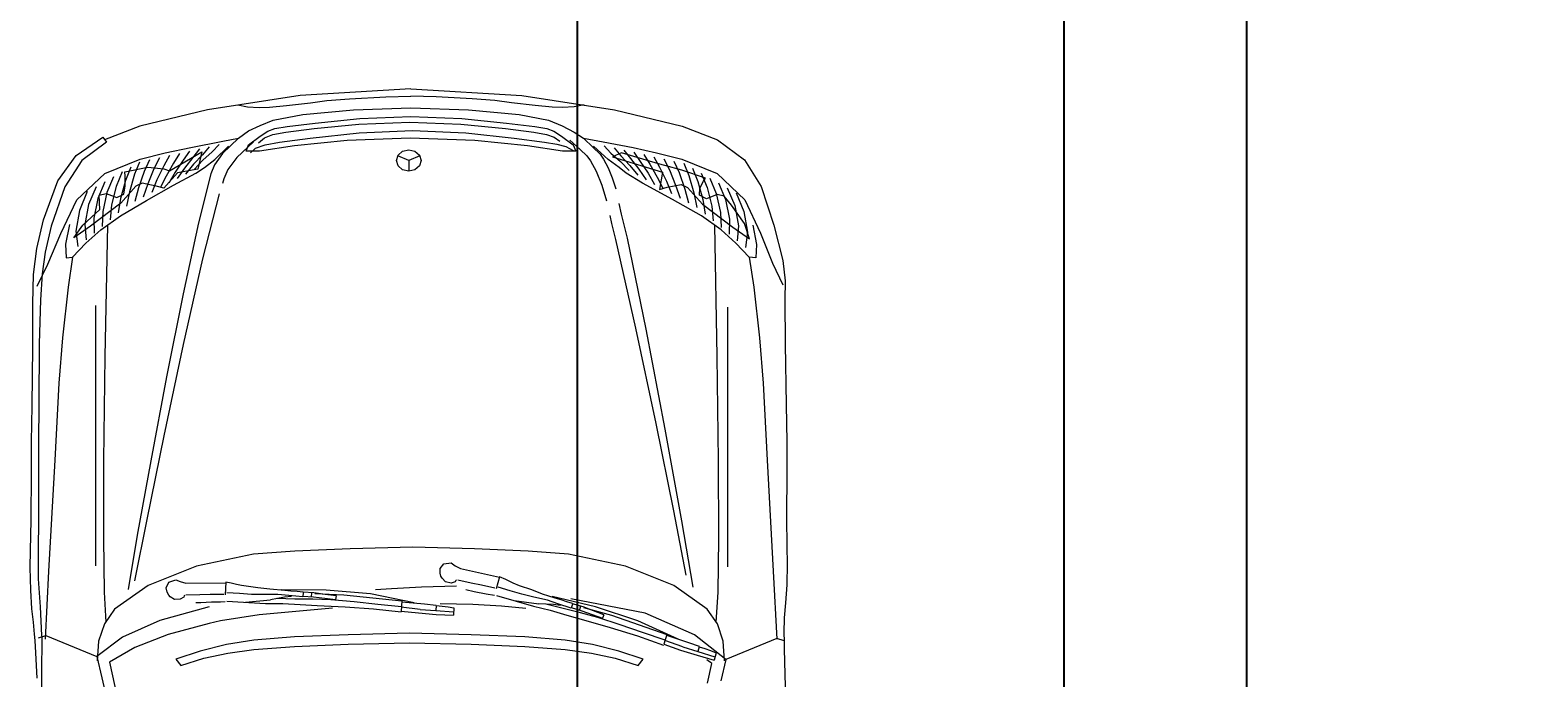
# Model space of a CAD drawing. Units: inches. Extents: x 37 to 706, y -568 to 110.
# Tile 14 of 24: x 452 to 526, y -405 to -373. Entities that reach past the tile are written whole.
import ezdxf

# ---------------------------------------------------------------- set-up
doc = ezdxf.new("R2010")
doc.units = ezdxf.units.IN
doc.header["$MEASUREMENT"] = 0
doc.layers.add('A-ANNO-DIMS', color=2, linetype='Continuous', lineweight=18)
doc.layers.add('A-SITE-VEHI', color=8, linetype='Continuous', lineweight=13)
doc.styles.get("Standard").update_dxf_attribs({"font": 'arial.ttf'})
doc.dimstyles.get("Standard").update_dxf_attribs({"dimtxt": 0.18, "dimasz": 0.18, "dimexe": 0.18, "dimexo": 0.0625, "dimgap": 0.09, "dimtad": 0, "dimtih": 1, "dimtoh": 1, "dimdec": 0, "dimzin": 0, "dimdsep": 46, "dimlunit": 3, "dimtxsty": 'Standard', "dimcen": 0.09, "dimadec": 0, "dimazin": 0, "dimtfac": 1, "dimtdec": 0, "dimtofl": 0, "dimtmove": 0, "dimatfit": 3, "dimfxl": 1, "dimtolj": 1, "dimtzin": 0, "dimarcsym": 0})

# ---------------------------------------------------------------- blocks, each defined once
blk = doc.blocks.new('CAR-SEDAN-PLAN')
for p, q in [((16.648, 91.844), (12.074, 91.146)), ((15.977, 91.359), (17.154, 91.49)), ((22.11, 92.169), (16.648, 91.844)), ((17.154, 91.49), (17.965, 91.597)), ((17.965, 91.597), (19.087, 91.685)), ((19.087, 91.685), (20.868, 91.772)), ((20.868, 91.772), (22.11, 91.812)), ((22.11, 92.169), (27.571, 91.844)), ((23.351, 91.772), (22.11, 91.812)), ((25.132, 91.685), (23.351, 91.772)), ((26.254, 91.597), (25.132, 91.685)), ((27.066, 91.49), (26.254, 91.597)), ((28.242, 91.359), (27.066, 91.49)), ((27.571, 91.844), (32.145, 91.146)), ((12.074, 91.146), (8.74, 90.335)), ((13.57, 91.383), (14.057, 91.284)), ((14.057, 91.284), (14.632, 91.256)), ((14.632, 91.256), (15.142, 91.276)), ((15.142, 91.276), (15.977, 91.359)), ((15.321, 90.633), (16.772, 90.917)), ((16.772, 90.917), (19.278, 91.146)), ((19.278, 91.146), (22.11, 91.24)), ((19.597, 90.705), (22.11, 90.811)), ((22.11, 91.24), (24.942, 91.146)), ((22.11, 90.811), (24.623, 90.705)), ((24.942, 91.146), (27.448, 90.917)), ((27.448, 90.917), (28.898, 90.633)), ((29.077, 91.276), (28.242, 91.359)), ((29.588, 91.256), (29.077, 91.276)), ((30.162, 91.284), (29.588, 91.256)), ((30.649, 91.383), (30.162, 91.284)), ((32.145, 91.146), (35.48, 90.335)), ((8.74, 90.335), (6.996, 89.668)), ((13.606, 89.739), (14.1, 90.1)), ((14.1, 90.1), (14.675, 90.37)), ((14.675, 90.37), (15.321, 90.633)), ((14.678, 89.847), (15.057, 90.081)), ((15.057, 90.081), (15.401, 90.212)), ((15.292, 89.924), (15.945, 90.036)), ((15.401, 90.212), (16, 90.311)), ((15.945, 90.036), (17.338, 90.213)), ((16, 90.311), (17.394, 90.488)), ((17.142, 89.744), (19.563, 89.998)), ((17.338, 90.213), (19.542, 90.43)), ((17.394, 90.488), (19.597, 90.705)), ((19.542, 90.43), (22.055, 90.536)), ((19.563, 89.998), (22.192, 90.123)), ((22.055, 90.536), (24.568, 90.43)), ((22.192, 90.123), (24.809, 89.998)), ((24.568, 90.43), (26.771, 90.213)), ((24.623, 90.705), (26.826, 90.488)), ((24.809, 89.998), (27.204, 89.744)), ((26.771, 90.213), (28.165, 90.036)), ((26.826, 90.488), (28.22, 90.311)), ((28.165, 90.036), (28.798, 89.928)), ((28.22, 90.311), (28.818, 90.212)), ((28.818, 90.212), (29.163, 90.081)), ((28.898, 90.633), (29.564, 90.343)), ((29.163, 90.081), (29.542, 89.847)), ((29.564, 90.343), (30.157, 90.045)), ((30.157, 90.045), (30.614, 89.739)), ((35.48, 90.335), (37.224, 89.668)), ((5.601, 88.894), (6.92, 89.795)), ((7.094, 89.544), (5.88, 88.648)), ((6.92, 89.795), (7.094, 89.544)), ((9.997, 89.025), (11.251, 89.289)), ((11.251, 89.289), (12.829, 89.594)), ((12.166, 89.318), (11.835, 88.927)), ((12.657, 89.426), (12.315, 89.065)), ((12.434, 88.691), (13.106, 89.346)), ((13.606, 89.739), (12.814, 88.982)), ((12.829, 89.594), (13.606, 89.739)), ((14.353, 89.555), (13.524, 88.797)), ((13.977, 89.1), (14.105, 89.414)), ((14.105, 89.414), (14.678, 89.847)), ((14.202, 89.012), (14.451, 89.242)), ((14.451, 89.242), (14.927, 89.418)), ((14.587, 89.505), (14.885, 89.766)), ((16.373, 89.358), (14.642, 89.096)), ((14.885, 89.766), (15.292, 89.924)), ((14.927, 89.418), (15.632, 89.546)), ((15.632, 89.546), (17.142, 89.744)), ((18.969, 89.62), (16.373, 89.358)), ((22.074, 89.739), (18.969, 89.62)), ((25.258, 89.62), (22.074, 89.739)), ((27.858, 89.358), (25.258, 89.62)), ((27.204, 89.744), (28.701, 89.546)), ((29.577, 89.096), (27.858, 89.358)), ((28.701, 89.546), (29.312, 89.449)), ((28.798, 89.928), (29.18, 89.791)), ((29.18, 89.791), (29.461, 89.588)), ((29.312, 89.449), (29.741, 89.324)), ((29.542, 89.847), (30.115, 89.414)), ((29.741, 89.324), (30.104, 89.134)), ((29.953, 89.642), (30.45, 89.191)), ((30.115, 89.414), (30.243, 89.1)), ((30.614, 89.739), (31.103, 89.28)), ((30.614, 89.739), (31.589, 89.567)), ((31.103, 89.28), (31.434, 88.948)), ((31.832, 88.694), (31.114, 89.346)), ((31.589, 89.567), (33.068, 89.276)), ((31.634, 89.371), (31.976, 89.009)), ((32.125, 89.263), (32.456, 88.872)), ((33.068, 89.276), (34.222, 89.025)), ((37.224, 89.668), (38.558, 88.671)), ((4.688, 87.635), (5.601, 88.894)), ((5.88, 88.648), (5.034, 87.338)), ((7.007, 87.995), (8.748, 88.708)), ((8.729, 88.56), (8.478, 87.96)), ((8.748, 88.708), (9.997, 89.025)), ((9.22, 88.669), (8.958, 88.098)), ((9.711, 88.777), (9.438, 88.236)), ((10.202, 88.885), (9.917, 88.374)), ((10.397, 88.512), (10.036, 87.874)), ((10.205, 88.137), (11.803, 89.066)), ((10.693, 88.993), (10.397, 88.512)), ((10.876, 88.651), (10.488, 88.068)), ((11.184, 89.102), (10.876, 88.651)), ((11.356, 88.789), (10.94, 88.262)), ((11.675, 89.21), (11.356, 88.789)), ((11.835, 88.927), (11.391, 88.457)), ((11.843, 88.651), (11.413, 88.201)), ((11.803, 89.066), (11.608, 88.22)), ((12.315, 89.065), (11.843, 88.651)), ((11.93, 88.29), (12.434, 88.691)), ((12.814, 88.982), (12.414, 88.426)), ((13.524, 88.797), (13.084, 88.202)), ((14.642, 89.096), (13.977, 89.1)), ((21.403, 88.642), (21.485, 88.91)), ((21.485, 88.373), (21.403, 88.642)), ((22.006, 88.642), (21.465, 88.872)), ((21.485, 88.91), (21.701, 89.101)), ((21.701, 89.101), (22.006, 89.174)), ((22.006, 89.174), (22.31, 89.101)), ((22.546, 88.872), (22.006, 88.642)), ((22.006, 88.642), (22.006, 88.11)), ((22.31, 89.101), (22.527, 88.91)), ((22.527, 88.91), (22.609, 88.642)), ((22.609, 88.642), (22.527, 88.373)), ((30.243, 89.1), (29.577, 89.096)), ((30.45, 89.191), (30.787, 88.865)), ((30.787, 88.865), (30.971, 88.623)), ((30.971, 88.623), (31.247, 88.111)), ((31.434, 88.948), (31.614, 88.703)), ((31.614, 88.703), (31.841, 88.274)), ((32.384, 88.296), (31.832, 88.694)), ((31.976, 89.009), (32.448, 88.596)), ((32.488, 89.011), (32.052, 88.817)), ((32.052, 88.817), (34.523, 88.059)), ((32.448, 88.596), (32.878, 88.146)), ((32.456, 88.872), (32.9, 88.401)), ((34.313, 88.478), (32.488, 89.011)), ((32.616, 89.155), (32.935, 88.733)), ((32.935, 88.733), (33.351, 88.207)), ((33.107, 89.047), (33.415, 88.595)), ((33.415, 88.595), (33.803, 88.013)), ((33.598, 88.938), (33.895, 88.457)), ((34.089, 88.83), (34.374, 88.319)), ((34.222, 89.025), (35.471, 88.708)), ((34.58, 88.722), (34.854, 88.181)), ((35.071, 88.613), (35.333, 88.043)), ((35.471, 88.708), (37.213, 87.995)), ((35.562, 88.505), (35.813, 87.905)), ((38.558, 88.671), (39.379, 87.367)), ((5.638, 86.702), (7.007, 87.995)), ((7.439, 87.833), (7.12, 87.067)), ((7.869, 88.075), (7.573, 87.365)), ((8.004, 88.083), (9.141, 88.312)), ((8.018, 87.864), (8.004, 88.083)), ((8.02, 87.4), (8.018, 87.864)), ((8.299, 88.318), (8.025, 87.663)), ((8.478, 87.96), (8.23, 87.097)), ((8.958, 88.098), (8.681, 87.291)), ((9.438, 88.236), (9.133, 87.485)), ((9.141, 88.312), (9.918, 88.231)), ((9.917, 88.374), (9.585, 87.68)), ((10.036, 87.874), (9.745, 87.293)), ((9.918, 88.231), (10.205, 88.137)), ((10.59, 88.027), (9.93, 87.273)), ((10.488, 88.068), (10.162, 87.52)), ((10.405, 87.423), (11.498, 88.024)), ((10.94, 88.262), (10.579, 87.747)), ((11.608, 88.22), (10.59, 88.027)), ((11.391, 88.457), (10.996, 87.974)), ((11.498, 88.024), (11.93, 88.29)), ((12.237, 87.977), (11.632, 85.572)), ((12.414, 88.426), (12.237, 87.977)), ((13.084, 88.202), (12.881, 87.731)), ((21.701, 88.182), (21.485, 88.373)), ((22.006, 88.11), (21.701, 88.182)), ((22.31, 88.182), (22.006, 88.11)), ((22.527, 88.373), (22.31, 88.182)), ((31.247, 88.111), (31.528, 87.423)), ((31.841, 88.274), (32.036, 87.783)), ((32.036, 87.783), (32.207, 87.242)), ((32.722, 88.024), (32.384, 88.296)), ((33.526, 87.525), (32.722, 88.024)), ((32.9, 88.401), (33.295, 87.919)), ((33.351, 88.207), (33.712, 87.692)), ((33.803, 88.013), (34.129, 87.465)), ((33.895, 88.457), (34.255, 87.819)), ((34.255, 87.819), (34.546, 87.238)), ((34.633, 88.402), (34.313, 88.478)), ((34.523, 88.059), (34.362, 87.218)), ((34.374, 88.319), (34.706, 87.625)), ((35.469, 88.167), (34.633, 88.402)), ((34.854, 88.181), (35.158, 87.43)), ((35.333, 88.043), (35.61, 87.236)), ((36.639, 87.768), (35.469, 88.167)), ((35.813, 87.905), (36.062, 87.042)), ((35.992, 88.263), (36.266, 87.608)), ((36.422, 88.02), (36.718, 87.31)), ((36.533, 87.617), (36.639, 87.768)), ((36.852, 87.778), (37.171, 87.012)), ((37.213, 87.995), (38.581, 86.702)), ((3.994, 85.722), (4.688, 87.635)), ((5.034, 87.338), (4.368, 85.408)), ((6.149, 87.105), (5.761, 86.175)), ((6.579, 87.348), (6.214, 86.472)), ((7.009, 87.59), (6.667, 86.77)), ((6.735, 86.931), (7.077, 87.019)), ((7.12, 87.067), (6.91, 86.129)), ((7.077, 87.019), (7.607, 86.812)), ((7.573, 87.365), (7.35, 86.452)), ((8.025, 87.663), (7.79, 86.774)), ((8.54, 87.37), (7.797, 86.541)), ((7.943, 86.98), (8.02, 87.4)), ((8.23, 87.097), (8.076, 86.385)), ((8.681, 87.291), (8.494, 86.612)), ((8.851, 87.516), (8.54, 87.37)), ((9.545, 87.384), (8.851, 87.516)), ((9.133, 87.485), (8.911, 86.839)), ((9.062, 86.674), (10.405, 87.423)), ((9.585, 87.68), (9.328, 87.066)), ((9.93, 87.273), (9.545, 87.384)), ((12.655, 87.001), (11.831, 83.79)), ((12.881, 87.731), (12.809, 87.511)), ((31.528, 87.423), (31.755, 86.658)), ((35.014, 86.725), (33.526, 87.525)), ((34.362, 87.218), (34.746, 87.329)), ((34.706, 87.625), (34.963, 87.011)), ((34.746, 87.329), (35.44, 87.461)), ((35.158, 87.43), (35.38, 86.784)), ((35.44, 87.461), (35.751, 87.315)), ((35.61, 87.236), (35.798, 86.557)), ((35.751, 87.315), (36.494, 86.486)), ((36.062, 87.042), (36.215, 86.33)), ((36.266, 87.608), (36.501, 86.719)), ((36.348, 86.925), (36.363, 87.278)), ((36.363, 87.278), (36.533, 87.617)), ((36.718, 87.31), (36.941, 86.397)), ((37.171, 87.012), (37.381, 86.074)), ((37.282, 87.535), (37.624, 86.715)), ((37.712, 87.293), (38.077, 86.417)), ((38.142, 87.05), (38.53, 86.12)), ((39.379, 87.367), (40.01, 85.452)), ((4.843, 85.044), (5.638, 86.702)), ((6.214, 86.472), (6.031, 85.483)), ((7.797, 86.541), (6.303, 85.406)), ((6.667, 86.77), (6.471, 85.806)), ((6.761, 86.233), (6.735, 86.931)), ((7.35, 86.452), (7.28, 85.724)), ((7.607, 86.812), (7.943, 86.98)), ((7.79, 86.774), (7.678, 86.054)), ((7.782, 85.916), (9.062, 86.674)), ((32.36, 86.52), (32.484, 85.989)), ((36.437, 85.916), (35.014, 86.725)), ((36.684, 86.757), (36.348, 86.925)), ((36.494, 86.486), (37.989, 85.351)), ((36.501, 86.719), (36.613, 85.999)), ((37.214, 86.963), (36.684, 86.757)), ((36.941, 86.397), (37.011, 85.669)), ((37.557, 86.876), (37.214, 86.963)), ((37.923, 86.436), (37.557, 86.876)), ((37.624, 86.715), (37.821, 85.751)), ((38.567, 85.53), (37.923, 86.436)), ((38.077, 86.417), (38.26, 85.428)), ((38.581, 86.702), (39.352, 85.06)), ((3.655, 84.305), (3.994, 85.722)), ((5.761, 86.175), (5.591, 85.161)), ((5.921, 85.456), (6.761, 86.233)), ((6.471, 85.806), (6.484, 85.063)), ((6.814, 85.229), (7.782, 85.916)), ((6.91, 86.129), (6.882, 85.394)), ((11.632, 85.572), (10.878, 82.065)), ((31.915, 85.932), (32.007, 85.538)), ((32.007, 85.538), (32.098, 85.143)), ((32.484, 85.989), (32.641, 85.34)), ((37.406, 85.229), (36.437, 85.916)), ((37.381, 86.074), (37.409, 85.339)), ((37.821, 85.751), (37.807, 85.008)), ((38.53, 86.12), (38.7, 85.105)), ((38.805, 84.779), (38.567, 85.53)), ((4.368, 85.408), (4.064, 84.126)), ((4.207, 83.537), (4.843, 85.044)), ((5.266, 85.479), (5.072, 84.518)), ((5.486, 84.834), (5.921, 85.456)), ((6.303, 85.406), (5.486, 84.834)), ((5.591, 85.161), (5.688, 84.402)), ((6.031, 85.483), (6.086, 84.733)), ((6.083, 84.566), (6.814, 85.229)), ((7.139, 85.452), (7.018, 78.984)), ((32.098, 85.143), (32.191, 84.749)), ((32.641, 85.34), (32.766, 84.808)), ((32.766, 84.808), (33.695, 80.324)), ((37.081, 85.452), (37.201, 78.984)), ((38.137, 84.566), (37.406, 85.229)), ((37.989, 85.351), (38.805, 84.779)), ((38.26, 85.428), (38.205, 84.678)), ((38.7, 85.105), (38.604, 84.347)), ((38.964, 85.445), (39.149, 84.498)), ((39.352, 85.06), (39.944, 83.583)), ((40.01, 85.452), (40.443, 83.712)), ((3.488, 83.013), (3.655, 84.305)), ((4.064, 84.126), (3.924, 83.058)), ((5.072, 84.518), (5.102, 83.849)), ((5.424, 83.88), (6.083, 84.566)), ((32.191, 84.749), (33.187, 80.374)), ((38.796, 83.88), (38.137, 84.566)), ((39.149, 84.498), (39.115, 83.845)), ((3.673, 82.45), (4.207, 83.537)), ((5.102, 83.849), (5.424, 83.88)), ((5.424, 83.88), (5.2, 82.403)), ((11.831, 83.79), (10.879, 79.575)), ((38.796, 83.88), (39.019, 82.403)), ((39.115, 83.845), (38.796, 83.88)), ((39.944, 83.583), (40.454, 82.512)), ((40.443, 83.712), (40.566, 82.702)), ((3.471, 81.595), (3.488, 83.013)), ((3.924, 83.058), (3.838, 81.777)), ((40.566, 82.702), (40.546, 81.772)), ((5.2, 82.403), (4.921, 79.902)), ((10.878, 82.065), (10.063, 77.979)), ((39.019, 82.403), (39.298, 79.902)), ((3.469, 79.46), (3.471, 81.595)), ((3.838, 81.777), (3.783, 79.595)), ((6.575, 68.65), (6.575, 81.495)), ((37.735, 68.611), (37.735, 81.405)), ((40.546, 81.772), (40.558, 79.591)), ((33.187, 80.374), (34.19, 75.667)), ((33.695, 80.324), (34.635, 75.398)), ((3.783, 79.595), (3.753, 76.594)), ((4.921, 79.902), (4.745, 77.663)), ((10.879, 79.575), (9.92, 75.059)), ((39.298, 79.902), (39.474, 77.663)), ((40.558, 79.591), (40.618, 76.592)), ((3.427, 76.546), (3.469, 79.46)), ((7.018, 78.984), (6.954, 73.857)), ((37.201, 78.984), (37.265, 73.857)), ((4.745, 77.663), (4.545, 73.869)), ((10.063, 77.979), (9.279, 73.84)), ((39.474, 77.663), (39.674, 73.869)), ((3.753, 76.594), (3.743, 74.768)), ((40.618, 76.592), (40.653, 74.768)), ((3.401, 74.768), (3.427, 76.546)), ((34.19, 75.667), (35.061, 71.363)), ((34.635, 75.398), (35.451, 70.877)), ((3.394, 73.244), (3.401, 74.768)), ((3.743, 74.768), (3.745, 73.25)), ((9.92, 75.059), (9.08, 70.94)), ((40.653, 74.768), (40.646, 73.29)), ((4.545, 73.869), (4.242, 68.391)), ((6.954, 73.857), (6.943, 70.006)), ((9.279, 73.84), (8.614, 70.171)), ((37.265, 73.857), (37.276, 70.006)), ((39.674, 73.869), (39.977, 68.391)), ((3.374, 70.909), (3.394, 73.244)), ((3.745, 73.25), (3.741, 70.929)), ((40.646, 73.29), (40.638, 71.042)), ((3.343, 69.409), (3.374, 70.909)), ((3.741, 70.929), (3.719, 69.434)), ((9.08, 70.94), (8.479, 67.921)), ((35.061, 71.363), (35.662, 68.196)), ((35.451, 70.877), (36.007, 67.608)), ((40.638, 71.042), (40.653, 69.588)), ((6.943, 70.006), (6.982, 67.366)), ((8.614, 70.171), (8.158, 67.498)), ((37.276, 70.006), (37.237, 67.366)), ((3.33, 68.57), (3.343, 69.409)), ((3.719, 69.434), (3.721, 68.015)), ((14.339, 69.23), (11.529, 68.645)), ((16.386, 69.388), (14.339, 69.23)), ((19.12, 69.493), (16.386, 69.388)), ((22.208, 69.572), (19.12, 69.493)), ((25.245, 69.493), (22.208, 69.572)), ((27.884, 69.388), (25.245, 69.493)), ((29.881, 69.23), (27.884, 69.388)), ((32.691, 68.645), (29.881, 69.23)), ((40.653, 69.588), (40.667, 68.779)), ((3.357, 67.456), (3.33, 68.57)), ((11.529, 68.645), (9.151, 67.695)), ((23.545, 68.289), (23.551, 68.52)), ((23.551, 68.52), (23.735, 68.76)), ((23.735, 68.76), (24.097, 68.799)), ((24.097, 68.799), (24.299, 68.657)), ((24.299, 68.657), (24.546, 68.526)), ((24.546, 68.526), (26.473, 68.092)), ((35.069, 67.695), (32.691, 68.645)), ((40.667, 68.779), (40.64, 67.717)), ((3.721, 68.015), (3.826, 66.632)), ((4.242, 68.391), (4.066, 65.05)), ((9.151, 67.695), (7.496, 66.515)), ((10.038, 67.577), (10.163, 67.852)), ((10.163, 67.852), (10.507, 67.971)), ((10.507, 67.971), (10.736, 67.879)), ((10.736, 67.879), (11.007, 67.807)), ((11.007, 67.807), (12.981, 67.817)), ((12.984, 67.849), (12.948, 67.224)), ((13.239, 67.799), (12.984, 67.849)), ((13.505, 67.735), (13.239, 67.799)), ((13.761, 67.687), (13.505, 67.735)), ((14.556, 67.58), (13.761, 67.687)), ((23.59, 68.141), (23.545, 68.289)), ((23.648, 68.043), (23.59, 68.141)), ((23.818, 67.872), (23.648, 68.043)), ((24.099, 67.811), (23.818, 67.872)), ((24.296, 67.875), (24.099, 67.811)), ((24.325, 67.935), (24.296, 67.875)), ((24.361, 67.962), (24.325, 67.935)), ((25.085, 67.81), (24.416, 67.948)), ((25.584, 67.703), (25.085, 67.81)), ((26.251, 67.559), (25.584, 67.703)), ((26.483, 68.122), (26.307, 67.522)), ((26.786, 67.983), (26.483, 68.122)), ((27.155, 67.801), (26.786, 67.983)), ((27.463, 67.673), (27.155, 67.801)), ((28.075, 67.467), (27.463, 67.673)), ((36.723, 66.515), (35.069, 67.695)), ((39.977, 68.391), (40.153, 65.05)), ((40.64, 67.717), (40.582, 66.836)), ((3.416, 66.545), (3.357, 67.456)), ((6.982, 67.366), (7.068, 65.872)), ((10.084, 67.351), (10.038, 67.577)), ((10.162, 67.216), (10.084, 67.351)), ((10.239, 67.134), (10.162, 67.216)), ((10.444, 67.005), (10.239, 67.134)), ((10.732, 67.009), (10.444, 67.005)), ((10.909, 67.115), (10.732, 67.009)), ((10.924, 67.181), (10.909, 67.115)), ((10.952, 67.215), (10.924, 67.181)), ((11.692, 67.23), (11.009, 67.214)), ((12.202, 67.238), (11.692, 67.23)), ((12.885, 67.248), (12.202, 67.238)), ((13.653, 67.289), (13.037, 67.33)), ((14.246, 67.249), (13.653, 67.289)), ((13.945, 66.863), (15.177, 66.982)), ((14.864, 67.243), (14.246, 67.249)), ((15.155, 67.5), (14.556, 67.58)), ((15.54, 67.244), (14.864, 67.243)), ((15.898, 67.437), (15.155, 67.5)), ((15.525, 67.047), (15.177, 66.982)), ((16.386, 67.022), (15.503, 67.047)), ((15.873, 67.117), (15.525, 67.047)), ((16.088, 67.199), (15.54, 67.244)), ((17.922, 67.462), (15.723, 67.48)), ((16.224, 67.141), (15.873, 67.117)), ((16.194, 67.415), (15.898, 67.437)), ((16.776, 67.124), (16.088, 67.199)), ((16.497, 67.388), (16.194, 67.415)), ((17.269, 67.011), (16.386, 67.022)), ((16.792, 67.365), (16.497, 67.388)), ((16.766, 67.163), (17.31, 67.127)), ((16.797, 67.346), (16.776, 67.124)), ((17.329, 67.319), (16.785, 67.353)), ((17.204, 67.326), (17.186, 67.136)), ((18.152, 66.977), (17.269, 67.011)), ((17.31, 67.127), (17.856, 67.065)), ((17.876, 67.251), (17.329, 67.319)), ((17.365, 67.301), (18.795, 67.235)), ((17.856, 67.065), (18.396, 66.992)), ((18.416, 67.172), (17.876, 67.251)), ((20.11, 67.269), (17.922, 67.462)), ((19.315, 66.878), (18.152, 66.977)), ((18.416, 67.172), (18.386, 66.99)), ((18.795, 67.235), (20.227, 67.083)), ((22.264, 66.832), (20.11, 67.269)), ((20.227, 67.083), (21.653, 66.928)), ((21.152, 67.521), (20.364, 67.481)), ((22.637, 67.604), (21.152, 67.521)), ((21.653, 66.928), (21.624, 66.426)), ((24.36, 67.655), (22.637, 67.604)), ((24.813, 67.489), (25.236, 67.39)), ((25.236, 67.39), (25.817, 67.28)), ((25.817, 67.28), (26.231, 67.207)), ((26.322, 67.197), (28.153, 66.664)), ((27.008, 67.427), (26.417, 67.605)), ((27.578, 67.254), (27.008, 67.427)), ((27.197, 66.945), (28.425, 66.784)), ((28.178, 67.109), (27.578, 67.254)), ((28.604, 67.264), (28.075, 67.467)), ((28.837, 66.958), (28.178, 67.109)), ((29.229, 67.066), (28.604, 67.264)), ((29.361, 66.791), (28.837, 66.958)), ((31.207, 66.635), (29.068, 67.147)), ((29.514, 66.981), (29.229, 67.066)), ((29.802, 66.885), (29.514, 66.981)), ((33.664, 66.317), (29.991, 67.029)), ((37.237, 67.366), (37.152, 65.872)), ((3.49, 65.874), (3.416, 66.545)), ((3.826, 66.632), (3.887, 65.216)), ((7.496, 66.515), (6.998, 65.803)), ((12.165, 66.636), (9.728, 65.963)), ((11.499, 66.856), (11.754, 66.85)), ((11.754, 66.85), (12.013, 66.864)), ((12.013, 66.864), (12.269, 66.878)), ((12.269, 66.878), (12.494, 66.885)), ((12.494, 66.885), (12.72, 66.89)), ((12.72, 66.89), (12.945, 66.9)), ((14.625, 66.238), (12.721, 65.94)), ((13.035, 66.911), (14.939, 66.803)), ((18.234, 66.568), (14.625, 66.238)), ((14.939, 66.803), (15.789, 66.795)), ((15.789, 66.795), (16.643, 66.752)), ((16.643, 66.752), (17.493, 66.701)), ((17.493, 66.701), (18.865, 66.631)), ((18.865, 66.631), (20.259, 66.538)), ((20.476, 66.753), (19.315, 66.878)), ((20.259, 66.538), (21.624, 66.384)), ((21.638, 66.636), (20.476, 66.753)), ((21.624, 66.426), (22.487, 66.333)), ((22.566, 66.509), (21.631, 66.624)), ((21.652, 66.887), (22.219, 66.829)), ((22.219, 66.829), (22.786, 66.779)), ((22.487, 66.333), (23.347, 66.265)), ((22.566, 66.509), (23.333, 66.449)), ((22.786, 66.779), (23.353, 66.722)), ((23.357, 66.702), (23.333, 66.449)), ((23.333, 66.449), (24.216, 66.384)), ((23.347, 66.265), (24.213, 66.218)), ((23.357, 66.702), (23.648, 66.671)), ((25.16, 66.751), (23.552, 66.78)), ((23.648, 66.671), (23.94, 66.635)), ((23.94, 66.635), (24.229, 66.594)), ((24.229, 66.594), (24.213, 66.218)), ((26.574, 66.668), (25.16, 66.751)), ((27.773, 66.553), (26.574, 66.668)), ((28.153, 66.664), (28.979, 66.465)), ((28.778, 66.769), (28.425, 66.784)), ((29.611, 66.552), (28.756, 66.774)), ((29.133, 66.759), (28.778, 66.769)), ((28.979, 66.465), (29.801, 66.23)), ((29.481, 66.704), (29.133, 66.759)), ((30.014, 66.563), (29.361, 66.791)), ((30.469, 66.342), (29.611, 66.552)), ((29.801, 66.23), (30.618, 65.99)), ((30.085, 66.794), (29.802, 66.885)), ((30.085, 66.774), (30.014, 66.563)), ((30.014, 66.603), (30.535, 66.446)), ((30.597, 66.628), (30.074, 66.784)), ((30.477, 66.664), (30.416, 66.483)), ((31.322, 66.11), (30.469, 66.342)), ((30.535, 66.446), (31.054, 66.263)), ((31.115, 66.439), (30.597, 66.628)), ((30.628, 66.603), (32.006, 66.218)), ((31.054, 66.263), (31.563, 66.07)), ((31.624, 66.241), (31.115, 66.439)), ((33.296, 65.954), (31.207, 66.635)), ((31.624, 66.241), (31.553, 66.07)), ((32.006, 66.218), (33.368, 65.747)), ((36.098, 65.263), (33.664, 66.317)), ((37.222, 65.803), (36.723, 66.515)), ((40.582, 66.836), (40.524, 66.091)), ((3.553, 65.288), (3.49, 65.874)), ((6.998, 65.803), (6.705, 64.942)), ((9.728, 65.963), (7.877, 65.137)), ((12.165, 65.811), (10.134, 65.275)), ((12.721, 65.94), (12.165, 65.811)), ((30.618, 65.99), (31.939, 65.612)), ((32.433, 65.752), (31.322, 66.11)), ((31.939, 65.612), (33.276, 65.209)), ((33.537, 65.369), (32.433, 65.752)), ((35.296, 65.044), (33.296, 65.954)), ((33.368, 65.747), (34.723, 65.275)), ((37.515, 64.942), (37.222, 65.803)), ((40.524, 66.091), (40.497, 65.354)), ((3.583, 64.975), (3.553, 65.288)), ((3.614, 64.361), (3.583, 64.975)), ((3.746, 65.115), (4.101, 65.222)), ((3.887, 65.216), (3.9, 65.188)), ((3.903, 64.803), (3.894, 63.679)), ((3.9, 65.188), (3.908, 65.155)), ((3.911, 65.118), (3.903, 64.803)), ((3.908, 65.155), (3.911, 65.118)), ((4.101, 65.222), (6.623, 64.191)), ((7.877, 65.137), (6.623, 64.191)), ((6.705, 64.942), (6.639, 63.978)), ((10.134, 65.275), (8.491, 64.633)), ((13.014, 64.773), (11.719, 64.455)), ((14.37, 64.993), (13.014, 64.773)), ((16.366, 65.151), (14.37, 64.993)), ((19.006, 65.255), (16.366, 65.151)), ((16.366, 64.684), (19.006, 64.788)), ((22.043, 65.335), (19.006, 65.255)), ((19.006, 64.788), (22.043, 64.867)), ((25.08, 65.255), (22.043, 65.335)), ((22.043, 64.867), (25.08, 64.788)), ((27.719, 65.151), (25.08, 65.255)), ((25.08, 64.788), (27.719, 64.684)), ((29.716, 64.993), (27.719, 65.151)), ((31.072, 64.773), (29.716, 64.993)), ((32.366, 64.455), (31.072, 64.773)), ((33.276, 65.209), (34.572, 64.752)), ((34.642, 64.993), (33.537, 65.369)), ((34.723, 65.275), (34.582, 64.792)), ((34.582, 64.792), (35.401, 64.507)), ((35.517, 64.662), (34.632, 64.983)), ((34.713, 65.235), (35.252, 65.051)), ((35.252, 65.051), (35.793, 64.875)), ((35.793, 64.875), (36.332, 64.692)), ((37.632, 64.039), (36.098, 65.263)), ((37.581, 63.978), (37.515, 64.942)), ((40.154, 65.07), (37.632, 64.039)), ((40.509, 64.963), (40.154, 65.07)), ((40.497, 65.354), (40.511, 64.943)), ((40.511, 64.943), (40.516, 64.555)), ((3.672, 63.126), (3.614, 64.361)), ((6.623, 64.191), (6.866, 63.136)), ((8.491, 64.633), (7.243, 63.902)), ((11.719, 64.455), (10.517, 64.056)), ((10.517, 64.056), (10.762, 63.739)), ((10.762, 63.739), (11.901, 64.099)), ((11.901, 64.099), (13.077, 64.344)), ((13.077, 64.344), (14.37, 64.526)), ((14.37, 64.526), (16.366, 64.684)), ((27.719, 64.684), (29.716, 64.526)), ((29.716, 64.526), (31.008, 64.344)), ((31.008, 64.344), (32.184, 64.099)), ((32.184, 64.099), (33.323, 63.739)), ((33.569, 64.056), (32.366, 64.455)), ((33.323, 63.739), (33.569, 64.056)), ((35.401, 64.507), (36.224, 64.248)), ((35.517, 64.662), (36.252, 64.43)), ((36.224, 64.248), (37.057, 64.008)), ((36.332, 64.672), (36.252, 64.43)), ((36.252, 64.43), (37.097, 64.168)), ((36.332, 64.672), (36.609, 64.576)), ((36.609, 64.576), (36.884, 64.475)), ((36.79, 63.963), (36.704, 64.018)), ((36.874, 63.902), (36.79, 63.963)), ((36.884, 64.475), (37.157, 64.37)), ((37.157, 64.37), (37.057, 64.008)), ((37.632, 64.039), (37.389, 62.984)), ((40.516, 64.555), (40.544, 63.318)), ((3.894, 63.679), (3.912, 61.483)), ((7.243, 63.902), (9.479, 53.69)), ((36.731, 62.877), (36.956, 63.837)), ((36.956, 63.837), (36.874, 63.902)), ((40.544, 63.318), (40.611, 61.119)), ((6.866, 63.136), (7.386, 60.866))]:
    blk.add_line(p, q)
blk = doc.blocks.new('*D53')
at = {"layer": 'A-ANNO-DIMS', "color": 0, "lineweight": -2, "transparency": 16777216}
for p, q in [((511.958, -151.771), (511.958, -567.638)), ((537.958, -151.771), (537.958, -567.638)), ((512.138, -567.458), (524.628, -567.458)), ((537.778, -567.458), (525.289, -567.458))]:
    blk.add_line(p, q, dxfattribs=at)
at = {"layer": 'A-ANNO-DIMS', "color": 0, "transparency": 16777216}
for points in [[(512.138, -567.428), (512.138, -567.488), (511.958, -567.458)], [(537.778, -567.428), (537.778, -567.488), (537.958, -567.458)]]:
    blk.add_solid(points, dxfattribs=at)
at = {"layer": 'Defpoints', "color": 0, "transparency": 16777216}
for p in [(511.958, -151.708), (537.958, -151.708), (537.958, -567.458)]:
    blk.add_point(p, dxfattribs=at)
at = {"layer": 'A-ANNO-DIMS', "color": 0, "transparency": 16777216, "insert": (524.958, -567.458), "char_height": 0.18, "attachment_point": 5}
blk.add_mtext('\\A1;2\'-2"', dxfattribs=at)
blk = doc.blocks.new('*D63')
at = {"layer": 'A-ANNO-DIMS', "color": 0, "lineweight": -2, "transparency": 16777216}
for p, q in [((478.958, -142.771), (478.958, -567.638)), ((502.958, -151.771), (502.958, -567.638)), ((479.138, -567.458), (490.628, -567.458)), ((502.778, -567.458), (491.289, -567.458))]:
    blk.add_line(p, q, dxfattribs=at)
at = {"layer": 'A-ANNO-DIMS', "color": 0, "transparency": 16777216}
for points in [[(479.138, -567.428), (479.138, -567.488), (478.958, -567.458)], [(502.778, -567.428), (502.778, -567.488), (502.958, -567.458)]]:
    blk.add_solid(points, dxfattribs=at)
at = {"layer": 'Defpoints', "color": 0, "transparency": 16777216}
for p in [(478.958, -142.708), (502.958, -151.708), (502.958, -567.458)]:
    blk.add_point(p, dxfattribs=at)
at = {"layer": 'A-ANNO-DIMS', "color": 0, "transparency": 16777216, "insert": (490.958, -567.458), "char_height": 0.18, "attachment_point": 5}
blk.add_mtext('\\A1;2\'-0"', dxfattribs=at)

msp = doc.modelspace()

# ---------------------------------------------------------------- block references
at = {"layer": 'A-SITE-VEHI'}
msp.add_blockref('CAR-SEDAN-PLAN', (448.648, -467.674), dxfattribs=at)

# ---------------------------------------------------------------- dimensions: what is measured, and where the dimension line sits
at = {"layer": 'A-ANNO-DIMS'}
for base, p1, p2, picture, middle in [((502.958, -567.458), (478.958, -142.708), (502.958, -151.708), '*D63', (490.958, -567.458)), ((537.958, -567.458), (511.958, -151.708), (537.958, -151.708), '*D53', (524.958, -567.458))]:
    dim = msp.add_linear_dim(base=base, p1=p1, p2=p2, dimstyle='Standard', override={"dimdec": 1, "dimlfac": 1, "dimrnd": 0, "dimzin": 1, "dimdsep": 46, "dimlunit": 4, "dimfrac": 2}, dxfattribs=at)
    dim.commit()
    dim.dimension.update_dxf_attribs({"geometry": picture, "text_midpoint": middle})

doc.saveas('drawing.dxf')
